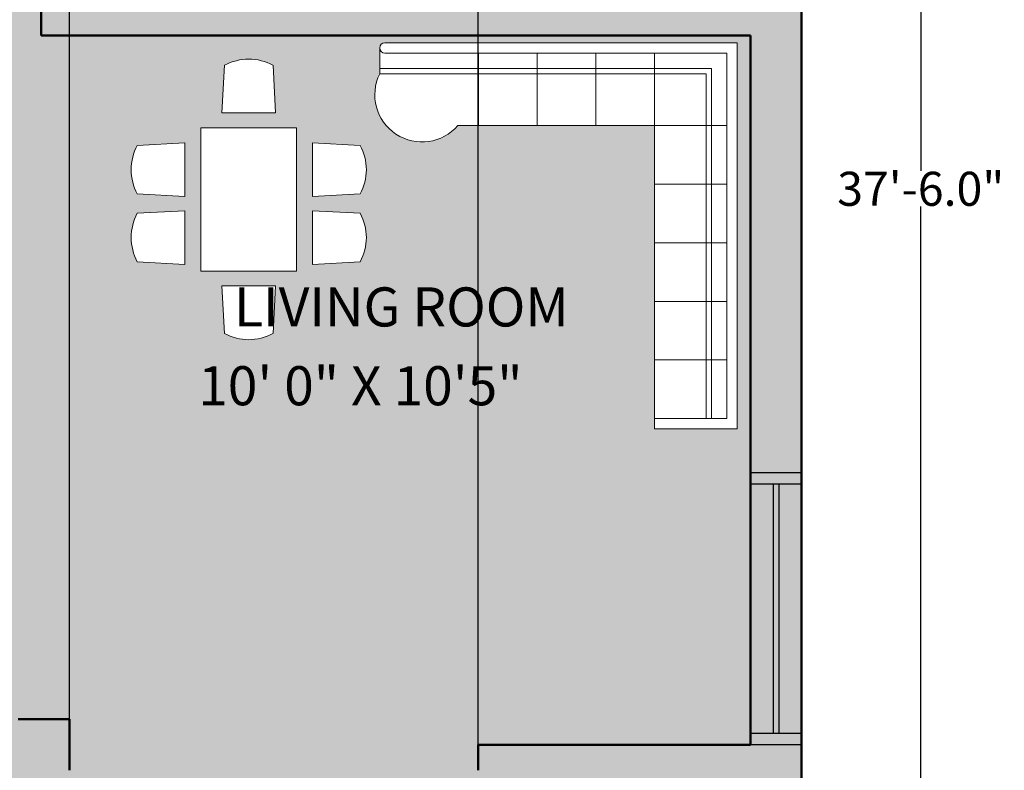
# Model space of a CAD drawing. Units: inches. Extents: x 528 to 2620, y -1066 to 798.
# Tile 24 of 41: x 1207 to 1381, y 391 to 524. Entities that reach past the tile are written whole.
import ezdxf

# ---------------------------------------------------------------- set-up
doc = ezdxf.new("R2010")
doc.units = ezdxf.units.IN
doc.header["$MEASUREMENT"] = 0
for name, color, linetype, lineweight in [('A-ANNO-DIMS', 2, 'Continuous', 18), ('A-AREA-IDEN', 7, 'Continuous', 18), ('A-FURN', 30, 'Continuous', 18), ('A-GLAZ', 3, 'Continuous', 25), ('A-WALL', 7, 'Continuous', 50), ('A-WALL-PATT', 8, 'Continuous', 13)]:
    doc.layers.add(name, color=color, linetype=linetype, lineweight=lineweight)
doc.styles.get("Standard").update_dxf_attribs({"font": 'arial.ttf'})
doc.dimstyles.get("Standard").update_dxf_attribs({"dimtxt": 6, "dimasz": 2, "dimexe": 0.18, "dimexo": 0.0625, "dimgap": 0.09, "dimtad": 0, "dimtih": 1, "dimtoh": 1, "dimdec": 1, "dimzin": 0, "dimdsep": 46, "dimlunit": 3, "dimtxsty": 'Standard', "dimblk": 'ARCHTICK', "dimcen": 0.09, "dimadec": 0, "dimazin": 0, "dimtfac": 1, "dimtdec": 1, "dimtofl": 0, "dimtmove": 0, "dimatfit": 3, "dimfxl": 1, "dimtolj": 1, "dimtzin": 0, "dimarcsym": 0})

# ---------------------------------------------------------------- blocks, each defined once
blk = doc.blocks.new('QU')
at = {"color": 0}
for p, q in [((-0.8, -2.5), (-0.8, 1.2333)), ((-0.8, 1.2333), (0, 1.2333)), ((0, 1.2333), (0, -2.4)), ((-0.7, -2.4), (-0.7, 1.1333)), ((-0.7, 1.1333), (0, 1.1333)), ((-0.55, -2.25), (-0.55, 1.1333)), ((-0.5, -2.2), (-0.5, 1.1333)), ((-0.7, 0.5666), (0, 0.5666)), ((-0.7, 0), (0, 0)), ((-0.7, -0.5667), (0, -0.5667)), ((-0.7, -1.1334), (0, -1.1334)), ((-0.7, -1.7), (1.1333, -1.7)), ((-0.1333, -1.7), (1.7, -1.7)), ((0.5667, -1.7), (0.5667, -2.4)), ((1.1333, -1.7), (1.1333, -2.4)), ((1.1334, -1.7), (1.1334, -2.4)), ((1.7, -1.7), (1.9, -1.7)), ((1.7, -1.7), (1.7, -2.4)), ((2.6553, -2.25), (-0.55, -2.25)), ((2.6553, -2.2), (-0.5, -2.2)), ((2.6553, -2.45), (2.6553, -2.2)), ((2.6053, -2.4), (-0.7, -2.4)), ((2.6053, -2.5), (-0.8, -2.5))]:
    blk.add_line(p, q, dxfattribs=at)
for centre, radius, start, end in [((2.2465, -1.9971), 0.4564, 333.59217, 139.39788), ((2.6053, -2.45), 0.05, 270, 90)]:
    blk.add_arc(centre, radius, start, end, dxfattribs=at)
blk = doc.blocks.new('table-11')
at = {"color": 0, "linetype": 'ByBlock'}
for p, q in [((-1.122, 0.5326), (-1.1442, 0.1341)), ((-0.7163, 0.5326), (-0.6942, 0.1341)), ((-0.5539, 0.5326), (-0.576, 0.1341)), ((-0.1482, 0.5326), (-0.126, 0.1341)), ((-1.1442, 0.1341), (-0.6942, 0.1341)), ((-0.576, 0.1341), (-0.126, 0.1341)), ((0, 0), (-1.2, 0)), ((-1.2, -0.8), (-1.2, 0)), ((0, -0.8), (0, 0)), ((-1.7227, -0.1971), (-1.3243, -0.175)), ((-1.3243, -0.625), (-1.3243, -0.175)), ((0.5227, -0.1971), (0.1243, -0.175)), ((0.1243, -0.625), (0.1243, -0.175)), ((-1.7227, -0.6029), (-1.3243, -0.625)), ((0.5227, -0.6029), (0.1243, -0.625)), ((0, -0.8), (-1.2, -0.8)), ((-1.1442, -0.9341), (-0.6942, -0.9341)), ((-1.122, -1.3326), (-1.1442, -0.9341)), ((-0.7163, -1.3326), (-0.6942, -0.9341)), ((-0.576, -0.9341), (-0.126, -0.9341)), ((-0.5539, -1.3326), (-0.576, -0.9341)), ((-0.1482, -1.3326), (-0.126, -0.9341))]:
    blk.add_line(p, q, dxfattribs=at)
for centre, start, end in [((-0.9192, 0.1591), 61.48912, 118.51088), ((-0.351, 0.1591), 61.48912, 118.51088), ((-1.3493, -0.4), 151.48912, 208.51088), ((0.1493, -0.4), 331.48912, 28.51088), ((-0.9192, -0.9591), 241.48912, 298.51088), ((-0.351, -0.9591), 241.48912, 298.51088)]:
    blk.add_arc(centre, 0.425, start, end, dxfattribs=at)
blk = doc.blocks.new('_ArchTick')
at = {"color": 0, "linetype": 'ByBlock', "const_width": 0.15}
blk.add_lwpolyline([(-0.5, -0.5), (0.5, 0.5)], dxfattribs=at)
blk = doc.blocks.new('*D17')
at = {"layer": 'A-ANNO-DIMS', "color": 0, "lineweight": -2, "transparency": 16777216}
for p, q in [((1345.06, 718.92), (1366.18, 718.92)), ((1366, 718.92), (1366, 497.08)), ((1366, 268.92), (1366, 490.77)), ((1345.06, 268.92), (1366.18, 268.92))]:
    blk.add_line(p, q, dxfattribs=at)
at = {"layer": 'Defpoints', "color": 0, "transparency": 16777216}
for p in [(1345, 718.92), (1345, 268.92), (1366, 268.92)]:
    blk.add_point(p, dxfattribs=at)
at = {"layer": 'A-ANNO-DIMS', "color": 0, "lineweight": -2, "transparency": 16777216, "xscale": 2, "yscale": 2, "zscale": 2}
for p, rotation in [((1366, 718.92), 90), ((1366, 268.92), 270)]:
    blk.add_blockref('_ArchTick', p, dxfattribs=dict(at, rotation=rotation))
at = {"layer": 'A-ANNO-DIMS', "color": 0, "transparency": 16777216, "insert": (1366, 493.92), "char_height": 6, "attachment_point": 5}
blk.add_mtext('\\A1;37\'-6.0"', dxfattribs=at)
blk = doc.blocks.new('WIN-1200')
for p, q in [((677.56, 718.92), (725.56, 718.92)), ((677.56, 709.92), (677.56, 718.92)), ((679.56, 709.92), (679.56, 718.92)), ((723.56, 718.92), (723.56, 709.92)), ((725.56, 718.92), (725.56, 709.92)), ((679.56, 714.92), (723.56, 714.92)), ((679.56, 713.92), (723.56, 713.92)), ((725.56, 709.92), (677.56, 709.92))]:
    blk.add_line(p, q)
blk = doc.blocks.new('*D68')
at = {"layer": 'A-ANNO-DIMS', "color": 0, "lineweight": -2, "transparency": 16777216}
for p, q in [((1216, 400.48), (1216, 751.1)), ((1216, 750.92), (1243.92, 750.92)), ((1288, 750.92), (1260.08, 750.92)), ((1288, 395.98), (1288, 751.1))]:
    blk.add_line(p, q, dxfattribs=at)
at = {"layer": 'Defpoints', "color": 0, "transparency": 16777216}
for p in [(1288, 750.92), (1216, 400.42), (1288, 395.92)]:
    blk.add_point(p, dxfattribs=at)
at = {"layer": 'A-ANNO-DIMS', "color": 0, "lineweight": -2, "transparency": 16777216, "xscale": 2, "yscale": 2, "zscale": 2, "rotation": 180}
blk.add_blockref('_ArchTick', (1216, 750.92), dxfattribs=at)
at = {"layer": 'A-ANNO-DIMS', "color": 0, "lineweight": -2, "transparency": 16777216, "xscale": 2, "yscale": 2, "zscale": 2}
blk.add_blockref('_ArchTick', (1288, 750.92), dxfattribs=at)
at = {"layer": 'A-ANNO-DIMS', "color": 0, "transparency": 16777216, "insert": (1252, 750.92), "char_height": 6, "attachment_point": 5}
blk.add_mtext('\\A1;6\'-0"', dxfattribs=at)

msp = doc.modelspace()

# ---------------------------------------------------------------- hatches: boundary and pattern name
at = {"layer": 'A-WALL-PATT', "transparency": 33554521}
h = msp.add_hatch(color=256, dxfattribs=at)
h.dxf.hatch_style = 1
h.paths.add_polyline_path([(1066, 709.92), (1114.5, 709.92), (1114.5, 718.92), (1057, 718.92), (1057, 667.92), (1066, 667.92)])
h.paths.add_polyline_path([(1227.5, 718.92), (1162.5, 718.92), (1162.5, 709.92), (1211, 709.92), (1211, 577.92), (1205.42, 577.92), (1205.5, 573.42), (1211, 573.42), (1211, 567.42), (1215.5, 567.42), (1215.5, 669.42), (1268, 669.42), (1268, 675.92), (1263.5, 675.92), (1263.5, 673.92), (1215.5, 673.92), (1215.5, 709.92), (1227.5, 709.92)])
h.paths.add_polyline_path([(1345, 718.92), (1316, 718.92), (1316, 709.92), (1336, 709.92), (1336, 641.67), (1345, 641.67)])
h.paths.add_polyline_path([(1066, 619.92), (1057, 619.92), (1057, 561.42), (1066, 561.42), (1066, 573.42), (1161, 573.42), (1161, 569.42), (1165.5, 569.42), (1165.5, 577.92), (1066, 577.92)])
h.paths.add_polyline_path([(1216, 391.42), (1216, 400.42), (1207, 400.42), (1201, 400.42), (1201, 397.42), (1201, 391.42), (1207, 391.42), (1207, 268.92), (1252, 268.92), (1252, 277.92), (1216, 277.92), (1216, 359.77)])
h.paths.add_polyline_path([(1345, 395.92), (1336, 395.92), (1288, 395.92), (1288, 391.42), (1336, 391.42), (1336, 277.92), (1300, 277.92), (1300, 268.92), (1345, 268.92)])
h.paths.add_polyline_path([(1345, 593.67), (1336, 593.67), (1336, 525.42), (1215.5, 525.42), (1215.5, 527.17), (1211, 527.17), (1211, 520.92), (1336, 520.92), (1336, 443.92), (1345, 443.92)])
h.paths.add_polyline_path([(1066, 520.92), (1165.5, 520.92), (1165.5, 545.42), (1161, 545.42), (1161, 525.42), (1066, 525.42), (1066, 537.42), (1057, 537.42), (1057, 484.67), (1066, 484.67)])
h.paths.add_polyline_path([(1066, 436.67), (1057, 436.67), (1057, 391.42), (1085.5, 391.42), (1085.5, 400.42), (1066, 400.42)])
h.paths.add_polyline_path([(1153, 397.42), (1153, 400.42), (1133.5, 400.42), (1133.5, 391.42), (1153, 391.42)])
at = {"layer": 'A-WALL-PATT', "transparency": 33554681}
h = msp.add_hatch(color=256, dxfattribs=at)
h.dxf.hatch_style = 1
h.paths.add_polyline_path([(1066, 665.92), (1062, 665.92), (1062, 621.92), (1066, 621.92)])
h.paths.add_polyline_path([(1061, 665.92), (1057, 665.92), (1057, 621.92), (1061, 621.92)])
h.paths.add_polyline_path([(1160.5, 713.92), (1116.5, 713.92), (1116.5, 709.92), (1160.5, 709.92)])
h.paths.add_polyline_path([(1160.5, 718.92), (1116.5, 718.92), (1116.5, 714.92), (1160.5, 714.92)])
h.paths.add_polyline_path([(1251.5, 713.92), (1227.5, 713.92), (1227.5, 709.92), (1251.5, 709.92)])
h.paths.add_polyline_path([(1251.5, 718.92), (1227.5, 718.92), (1227.5, 714.92), (1251.5, 714.92)])
h.paths.add_polyline_path([(1314, 713.92), (1270, 713.92), (1270, 709.92), (1314, 709.92)])
h.paths.add_polyline_path([(1314, 718.92), (1270, 718.92), (1270, 714.92), (1314, 714.92)])
h.paths.add_polyline_path([(1345, 639.67), (1341, 639.67), (1341, 595.67), (1345, 595.67)])
h.paths.add_polyline_path([(1340, 639.67), (1336, 639.67), (1336, 595.67), (1340, 595.67)])
h.paths.add_polyline_path([(1345, 441.92), (1341, 441.92), (1341, 397.92), (1345, 397.92)])
h.paths.add_polyline_path([(1340, 441.92), (1336, 441.92), (1336, 397.92), (1340, 397.92)])
h.paths.add_polyline_path([(1298, 272.92), (1254, 272.92), (1254, 268.92), (1298, 268.92)])
h.paths.add_polyline_path([(1298, 277.92), (1254, 277.92), (1254, 273.92), (1298, 273.92)])
h.paths.add_polyline_path([(1131.5, 395.42), (1087.5, 395.42), (1087.5, 391.42), (1131.5, 391.42)])
h.paths.add_polyline_path([(1131.5, 400.42), (1087.5, 400.42), (1087.5, 396.42), (1131.5, 396.42)])
h.paths.add_polyline_path([(1066, 482.67), (1062, 482.67), (1062, 438.67), (1066, 438.67)])
h.paths.add_polyline_path([(1061, 482.67), (1057, 482.67), (1057, 438.67), (1061, 438.67)])
h.paths.add_polyline_path([(1066, 561.42), (1062, 561.42), (1062, 537.42), (1066, 537.42)])
h.paths.add_polyline_path([(1061, 561.42), (1057, 561.42), (1057, 537.42), (1061, 537.42)])
at = {"layer": 'A-WALL-PATT', "transparency": 33554536}
h = msp.add_hatch(color=256, dxfattribs=at)
h.dxf.hatch_style = 1
h.paths.add_polyline_path([(1336, 709.92), (1268, 709.92), (1268, 699.92), (1266.75, 699.92), (1266.75, 675.92), (1268, 675.92), (1268, 669.42), (1215.5, 669.42), (1215.5, 567.17), (1217, 567.17), (1257, 567.17), (1257, 565.42), (1256.96, 565.42, -0.401453), (1217, 527.17), (1215.5, 527.17), (1215.5, 525.42), (1336, 525.42)], flags=17)
h.paths.add_polyline_path([(1285.03, 635.93), (1285.23, 636.13), (1285.67, 636.26), (1286.21, 636.02), (1286.98, 636.08), (1332.98, 636.08), (1333.36, 636.22), (1333.82, 636.08), (1334.11, 635.71), (1334.11, 635.3), (1333.91, 634.86), (1333.82, 634.83), (1333.82, 592.74), (1333.97, 592.6), (1334.11, 592.29), (1334.11, 591.88), (1333.82, 591.51), (1333.36, 591.37), (1332.98, 591.51), (1332.64, 591.79), (1332.64, 591.51), (1286.98, 591.51), (1286.17, 591.67), (1286.07, 591.57), (1285.68, 591.37), (1285.23, 591.51), (1285.03, 591.71), (1284.83, 592.1), (1284.98, 592.54), (1285.13, 592.69), (1285.13, 634.95), (1284.98, 635.1), (1284.83, 635.54)], flags=16)
h.paths.add_polyline_path([(1285.03, 635.93), (1285.23, 636.13), (1285.67, 636.26), (1286.21, 636.02), (1286.98, 636.08), (1332.98, 636.08), (1333.36, 636.22), (1333.82, 636.08), (1334.11, 635.71), (1334.11, 635.3), (1333.97, 634.99), (1333.82, 634.85), (1333.82, 592.74), (1333.97, 592.6), (1334.11, 592.29), (1334.11, 591.88), (1333.82, 591.51), (1333.36, 591.37), (1332.98, 591.51), (1332.64, 591.79), (1332.64, 592.25), (1332.64, 635.35), (1332.64, 635.8), (1332.98, 636.08), (1312.23, 636.08), (1311.1, 635.48), (1310.63, 635.48), (1310.43, 635.23), (1309.94, 635.1), (1309.7, 634.99), (1309.06, 634.76), (1308.71, 634.61), (1308.32, 634.61), (1307.75, 634.36), (1307.11, 634.27), (1307.01, 634.11), (1306.77, 634.02), (1307.25, 633.28), (1306.87, 633.04), (1306.77, 632.88), (1306.37, 632.64), (1306.03, 632.55), (1305.54, 632.41), (1315.47, 618.49), (1316.32, 619.39), (1312.77, 622.86), (1319.62, 630.11), (1320.07, 629.68), (1320.11, 630), (1320.28, 630.6), (1320.53, 631.18), (1320.53, 632.01), (1320.26, 632.55), (1320.11, 633.13), (1320.06, 633.73), (1320.63, 634.02), (1321.22, 634.16), (1321.86, 634.11), (1322.45, 633.91), (1322.99, 633.62), (1324.1, 633.62), (1324.64, 633.91), (1325.23, 634.07), (1325.87, 634.07), (1326.43, 633.91), (1326.98, 633.62), (1328.35, 633.62), (1328.9, 633.91), (1329.49, 634.11), (1330.1, 634.16), (1330.69, 634.02), (1331.28, 633.73), (1331.23, 633.13), (1331.09, 632.55), (1330.79, 632.01), (1330.79, 631.18), (1331.04, 630.6), (1331.23, 630), (1331.28, 629.41), (1331.19, 628.79), (1331.04, 628.18), (1330.79, 627.6), (1330.79, 626.77), (1331.04, 626.19), (1331.23, 625.59), (1331.28, 625.01), (1331.19, 624.38), (1331.04, 623.78), (1330.79, 623.24), (1330.79, 622.37), (1331.04, 621.83), (1331.23, 621.25), (1331.28, 620.6), (1331.19, 619.97), (1331.04, 619.37), (1330.79, 618.83), (1330.79, 617.96), (1331.09, 617.42), (1331.23, 616.88), (1331.28, 616.23), (1331.28, 615.52), (1330.69, 615.27), (1330.1, 615.12), (1329.49, 615.12), (1328.9, 615.32), (1328.35, 615.65), (1326.98, 615.65), (1326.43, 615.32), (1325.87, 615.16), (1325.23, 615.16), (1324.64, 615.32), (1324.1, 615.65), (1323.24, 615.65), (1324.93, 614.04), (1322.98, 611.98), (1324.1, 611.98), (1324.64, 612.27), (1325.28, 612.43), (1325.87, 612.43), (1326.48, 612.27), (1327.03, 611.98), (1328.35, 611.98), (1328.9, 612.27), (1329.49, 612.48), (1330.1, 612.52), (1330.74, 612.39), (1331.28, 612.07), (1331.28, 611.36), (1331.28, 610.75), (1331.09, 610.17), (1330.79, 609.63), (1330.79, 608.81), (1331.09, 608.22), (1331.23, 607.62), (1331.28, 606.99), (1331.23, 606.41), (1331.09, 605.81), (1330.79, 605.22), (1330.79, 604.4), (1331.09, 603.81), (1331.23, 603.21), (1331.28, 602.63), (1331.23, 602), (1331.09, 601.4), (1330.79, 600.86), (1330.79, 599.99), (1331.09, 599.45), (1331.23, 598.87), (1331.28, 598.22), (1331.23, 597.59), (1331.09, 596.99), (1330.79, 596.45), (1330.79, 595.58), (1331.09, 595.04), (1331.28, 594.51), (1331.28, 593.86), (1330.74, 593.61), (1330.1, 593.48), (1329.49, 593.48), (1328.9, 593.68), (1328.35, 594.01), (1327.03, 594.01), (1326.48, 593.68), (1325.87, 593.52), (1325.28, 593.52), (1324.64, 593.68), (1324.1, 594.01), (1323.04, 594.01), (1322.5, 593.68), (1321.91, 593.48), (1321.27, 593.48), (1320.63, 593.61), (1320.11, 593.86), (1320.11, 594.51), (1320.28, 595.04), (1320.58, 595.58), (1320.58, 596.45), (1320.28, 596.99), (1320.16, 597.59), (1320.1, 598.01), (1319.62, 597.55), (1315.66, 601.73), (1312.23, 591.57), (1311.74, 591.66), (1311.59, 591.91), (1310.78, 592.4), (1309.55, 592.89), (1308.96, 592.89), (1308.71, 593.03), (1308.56, 593.14), (1307.75, 593.52), (1306.77, 593.61), (1307.25, 594.36), (1306.87, 594.6), (1306.37, 594.84), (1306.03, 595.09), (1305.54, 595.24), (1315.46, 609.35), (1310.93, 613.71), (1315.47, 618.49), (1305.54, 632.41), (1306.03, 632.55), (1306.37, 632.64), (1306.77, 632.88), (1306.87, 633.04), (1307.25, 633.28), (1306.77, 634.02), (1307.01, 634.11), (1307.11, 634.27), (1307.75, 634.36), (1308.32, 634.61), (1308.71, 634.61), (1309.06, 634.76), (1309.7, 634.99), (1309.94, 635.1), (1310.43, 635.23), (1310.63, 635.48), (1311.1, 635.48), (1312.23, 636.08), (1286.98, 636.08), (1286.22, 636.02), (1286.41, 635.44), (1286.21, 635.05), (1286.02, 634.85), (1285.87, 634.81), (1285.87, 592.84), (1286.15, 592.73), (1286.41, 592.19), (1286.23, 591.66), (1286.17, 591.67), (1286.07, 591.57), (1285.68, 591.37), (1285.23, 591.51), (1285.03, 591.71), (1284.83, 592.1), (1284.98, 592.54), (1285.13, 592.69), (1285.13, 634.95), (1284.98, 635.1), (1284.83, 635.54)], flags=0)
h.paths.add_polyline_path([(1322.5, 653.6), (1333.65, 653.6), (1333.65, 637.99), (1322.5, 637.99)], flags=16)
h.paths.add_polyline_path([(1323.62, 652.48), (1332.53, 652.48), (1332.53, 639.11), (1323.62, 639.11)], flags=0)
edge = h.paths.add_edge_path(flags=0)
edge.add_ellipse((1328.07, 645.79), major_axis=(2.24, 2.24), ratio=1, start_angle=405, end_angle=495, ccw=False)
edge.add_ellipse((1328.07, 645.79), major_axis=(2.24, 2.24), ratio=1, start_angle=675, end_angle=765, ccw=False)
edge.add_ellipse((1328.07, 645.79), major_axis=(2.24, 2.24), ratio=1, start_angle=585, end_angle=675, ccw=False)
edge.add_ellipse((1328.07, 645.79), major_axis=(2.24, 2.24), ratio=1, start_angle=495, end_angle=585, ccw=False)
h.paths.add_polyline_path([(1320.58, 628.39), (1320.33, 628.01), (1320.61, 628.55)], flags=0)
h.paths.add_polyline_path([(1317.89, 604.89), (1318.78, 604.64), (1319.76, 604.28), (1318.88, 604.53)], flags=0)
h.paths.add_polyline_path([(1320.33, 599.65), (1320.58, 599.25), (1320.58, 599.16)], flags=0)
h.paths.add_polyline_path([(1322.5, 589.6), (1333.65, 589.6), (1333.65, 573.99), (1322.5, 573.99)], flags=16)
h.paths.add_polyline_path([(1323.62, 588.48), (1332.53, 588.48), (1332.53, 575.11), (1323.62, 575.11)], flags=0)
edge = h.paths.add_edge_path(flags=0)
edge.add_ellipse((1328.07, 581.8), major_axis=(-2.24, 2.24), ratio=1, start_angle=-45, end_angle=45, ccw=False)
edge.add_ellipse((1328.07, 581.8), major_axis=(-2.24, 2.24), ratio=1, start_angle=-135, end_angle=-45, ccw=False)
edge.add_ellipse((1328.07, 581.8), major_axis=(-2.24, 2.24), ratio=1, start_angle=135, end_angle=-135, ccw=False)
edge.add_ellipse((1328.07, 581.8), major_axis=(-2.24, 2.24), ratio=1, start_angle=45, end_angle=135, ccw=False)
h.paths.add_polyline_path([(1264.75, 699.92), (1263.5, 699.92), (1263.5, 709.92), (1215.5, 709.92), (1215.5, 673.92), (1263.5, 673.92), (1263.5, 675.92), (1264.75, 675.92)], flags=16)
h.paths.add_polyline_path([(1162.19, 569.42), (1161, 569.42), (1161, 573.42), (1066, 573.42), (1066, 525.42), (1161, 525.42), (1161, 545.42), (1162.19, 545.42)])
h.paths.add_polyline_path([(1256.96, 565.42), (1257, 565.42), (1257, 567.17), (1217, 567.17), (1215.5, 567.17), (1215.5, 567.42), (1211, 567.42), (1211, 573.42), (1205.5, 573.42), (1205.42, 577.92), (1211, 577.92), (1211, 709.92), (1066, 709.92), (1066, 577.92), (1165.5, 577.92), (1165.5, 569.42), (1164.19, 569.42), (1164.19, 545.42), (1165.5, 545.42), (1165.5, 520.92), (1153, 520.92), (1153, 484.92), (1102, 484.92), (1102, 436.42), (1153, 436.42), (1153, 400.42), (1153, 391.42), (1201, 391.42), (1201, 400.42), (1207, 400.42), (1216, 400.42), (1216, 391.42), (1216, 277.92), (1336, 277.92), (1336, 391.42), (1288, 391.42), (1288, 395.92), (1336, 395.92), (1336, 443.92), (1336, 520.92), (1211, 520.92), (1211, 527.17), (1215.5, 527.17), (1217, 527.17, 0.401453)])
h.paths.add_polyline_path([(1167.25, 579.42), (1165.5, 579.42), (1165.5, 619.42), (1167.25, 619.42)], flags=16)
h.paths.add_polyline_path([(1227.97, 501.56), (1236.36, 502.03), (1236.36, 492.55), (1227.97, 493.02, -0.254069)], flags=16)
h.paths.add_polyline_path([(1243.34, 515.69, -0.254069), (1251.88, 515.69), (1252.35, 507.3), (1242.87, 507.3)], flags=16)
h.paths.add_polyline_path([(1239.18, 504.68), (1256.03, 504.68), (1256.03, 479.42), (1239.18, 479.42)], flags=16)
h.paths.add_polyline_path([(1227.97, 489.6), (1236.36, 490.07), (1236.36, 480.59), (1227.97, 481.06, -0.254069)], flags=16)
h.paths.add_polyline_path([(1197.2, 624.04), (1197.2, 639.64), (1208.35, 639.64), (1208.35, 624.04)], flags=16)
h.paths.add_polyline_path([(1198.32, 625.15), (1198.32, 638.53), (1207.23, 638.53), (1207.23, 625.15)], flags=0)
h.paths.add_polyline_path([(1258.85, 502.03), (1267.25, 501.56, -0.254069), (1267.25, 493.02), (1258.85, 492.55)], flags=16)
h.paths.add_polyline_path([(1271.59, 519.66), (1333.67, 519.66), (1333.67, 451.59), (1319.09, 451.59), (1319.09, 505.07), (1288.09, 505.07), (1284.45, 505.07, -0.883215), (1270.68, 514.19), (1270.68, 518.75, -0.414214)], flags=16)
h.paths.add_polyline_path([(1331.85, 517.83), (1331.85, 453.42), (1328.2, 453.42), (1328.2, 505.07), (1298.42, 505.07), (1298.42, 514.19), (1288.09, 514.19), (1288.09, 517.83)], flags=0)
h.paths.add_polyline_path([(1242.87, 476.8), (1252.35, 476.8), (1251.88, 468.41, -0.254069), (1243.34, 468.41)], flags=16)
h.paths.add_polyline_path([(1258.85, 490.07), (1267.25, 489.6, -0.254069), (1267.25, 481.06), (1258.85, 480.59)], flags=16)
h.paths.add_polyline_path([(1161.68, 641.55), (1160.87, 641.72), (1160.77, 641.62), (1160.38, 641.41), (1159.93, 641.55), (1159.73, 641.75), (1159.53, 642.14), (1159.68, 642.58), (1159.83, 642.73), (1159.83, 684.99), (1159.68, 685.14), (1159.53, 685.58), (1159.73, 685.97), (1159.93, 686.17), (1160.37, 686.31), (1160.91, 686.06), (1161.68, 686.13), (1207.68, 686.13), (1208.06, 686.27), (1208.52, 686.13), (1208.81, 685.76), (1208.81, 685.34), (1208.61, 684.9), (1208.52, 684.87), (1208.52, 642.78), (1208.67, 642.65), (1208.88, 642.2), (1208.72, 641.8), (1208.52, 641.55), (1208.06, 641.41), (1207.68, 641.55), (1207.34, 641.83), (1207.34, 641.55)], flags=16)
h.paths.add_polyline_path([(1186.93, 641.62), (1186.44, 641.71), (1186.29, 641.95), (1185.48, 642.45), (1184.25, 642.94), (1183.66, 642.94), (1183.41, 643.07), (1183.26, 643.18), (1182.45, 643.57), (1181.47, 643.65), (1181.95, 644.4), (1181.57, 644.64), (1181.07, 644.89), (1180.73, 645.13), (1180.24, 645.29), (1190.16, 659.4), (1185.63, 663.75), (1190.17, 668.54), (1180.24, 682.46), (1180.73, 682.59), (1181.07, 682.68), (1181.47, 682.93), (1181.57, 683.08), (1181.95, 683.33), (1181.47, 684.07), (1181.71, 684.16), (1181.81, 684.31), (1182.45, 684.4), (1183.02, 684.65), (1183.41, 684.65), (1183.76, 684.81), (1184.4, 685.03), (1184.64, 685.14), (1185.13, 685.28), (1185.33, 685.52), (1185.8, 685.52), (1186.93, 686.13), (1161.68, 686.13), (1160.92, 686.06), (1161.11, 685.49), (1160.91, 685.1), (1160.72, 684.9), (1160.57, 684.85), (1160.57, 642.88), (1160.85, 642.77), (1161.11, 642.23), (1160.93, 641.7), (1160.87, 641.72), (1160.77, 641.62), (1160.38, 641.41), (1159.93, 641.55), (1159.73, 641.75), (1159.53, 642.14), (1159.68, 642.58), (1159.83, 642.73), (1159.83, 684.99), (1159.68, 685.14), (1159.53, 685.58), (1159.73, 685.97), (1159.93, 686.17), (1160.37, 686.31), (1160.91, 686.06), (1161.68, 686.13), (1207.68, 686.13), (1208.06, 686.27), (1208.52, 686.13), (1208.81, 685.76), (1208.81, 685.34), (1208.67, 685.03), (1208.52, 684.9), (1208.52, 642.78), (1208.67, 642.65), (1208.88, 642.2), (1208.72, 641.8), (1208.52, 641.55), (1208.06, 641.41), (1207.68, 641.55), (1207.34, 641.83), (1207.34, 642.29), (1207.34, 685.39), (1207.34, 685.85), (1207.68, 686.13), (1186.93, 686.13), (1185.8, 685.52), (1185.33, 685.52), (1185.13, 685.28), (1184.64, 685.14), (1184.4, 685.03), (1183.76, 684.81), (1183.41, 684.65), (1183.02, 684.65), (1182.45, 684.4), (1181.81, 684.31), (1181.71, 684.16), (1181.47, 684.07), (1181.95, 683.33), (1181.57, 683.08), (1181.47, 682.93), (1181.07, 682.68), (1180.73, 682.59), (1180.24, 682.46), (1190.17, 668.54), (1191.02, 669.43), (1187.47, 672.9), (1194.32, 680.15), (1194.77, 679.72), (1194.81, 680.04), (1194.98, 680.65), (1195.23, 681.23), (1195.23, 682.05), (1194.96, 682.59), (1194.81, 683.17), (1194.76, 683.78), (1195.33, 684.07), (1195.92, 684.2), (1196.56, 684.16), (1197.15, 683.96), (1197.69, 683.67), (1198.8, 683.67), (1199.34, 683.96), (1199.93, 684.11), (1200.57, 684.11), (1201.13, 683.96), (1201.68, 683.67), (1203.05, 683.67), (1203.6, 683.96), (1204.19, 684.16), (1204.8, 684.2), (1205.39, 684.07), (1205.98, 683.78), (1205.93, 683.17), (1205.79, 682.59), (1205.49, 682.05), (1205.49, 681.23), (1205.74, 680.65), (1205.93, 680.04), (1205.98, 679.46), (1205.89, 678.83), (1205.74, 678.23), (1205.49, 677.65), (1205.49, 676.82), (1205.74, 676.24), (1205.93, 675.63), (1205.98, 675.05), (1205.89, 674.42), (1205.74, 673.82), (1205.49, 673.28), (1205.49, 672.41), (1205.74, 671.87), (1205.93, 671.29), (1205.98, 670.64), (1205.89, 670.02), (1205.74, 669.41), (1205.49, 668.87), (1205.49, 668), (1205.79, 667.46), (1205.93, 666.93), (1205.98, 666.28), (1205.98, 665.56), (1205.39, 665.32), (1204.8, 665.16), (1204.19, 665.16), (1203.6, 665.36), (1203.05, 665.7), (1201.68, 665.7), (1201.13, 665.36), (1200.57, 665.2), (1199.93, 665.2), (1199.34, 665.36), (1198.8, 665.7), (1197.94, 665.7), (1199.63, 664.09), (1197.68, 662.03), (1198.8, 662.03), (1199.34, 662.32), (1199.98, 662.47), (1200.57, 662.47), (1201.18, 662.32), (1201.73, 662.03), (1203.05, 662.03), (1203.6, 662.32), (1204.19, 662.52), (1204.8, 662.56), (1205.44, 662.43), (1205.98, 662.12), (1205.98, 661.4), (1205.98, 660.8), (1205.79, 660.21), (1205.49, 659.68), (1205.49, 658.85), (1205.79, 658.27), (1205.93, 657.66), (1205.98, 657.04), (1205.93, 656.45), (1205.79, 655.85), (1205.49, 655.27), (1205.49, 654.44), (1205.79, 653.86), (1205.93, 653.25), (1205.98, 652.67), (1205.93, 652.05), (1205.79, 651.44), (1205.49, 650.91), (1205.49, 650.03), (1205.79, 649.5), (1205.93, 648.91), (1205.98, 648.26), (1205.93, 647.64), (1205.79, 647.03), (1205.49, 646.5), (1205.49, 645.62), (1205.79, 645.09), (1205.98, 644.55), (1205.98, 643.9), (1205.44, 643.65), (1204.8, 643.52), (1204.19, 643.52), (1203.6, 643.72), (1203.05, 644.06), (1201.73, 644.06), (1201.18, 643.72), (1200.57, 643.57), (1199.98, 643.57), (1199.34, 643.72), (1198.8, 644.06), (1197.74, 644.06), (1197.2, 643.72), (1196.61, 643.52), (1195.97, 643.52), (1195.33, 643.65), (1194.81, 643.9), (1194.81, 644.55), (1194.98, 645.09), (1195.28, 645.62), (1195.28, 646.5), (1194.98, 647.03), (1194.86, 647.64), (1194.8, 648.06), (1194.32, 647.59), (1190.36, 651.77)], flags=16)
h.paths.add_polyline_path([(1195.28, 649.2), (1195.03, 649.7), (1195.28, 649.29)], flags=0)
h.paths.add_polyline_path([(1194.46, 654.33), (1193.58, 654.58), (1192.59, 654.93), (1193.48, 654.69)], flags=0)
h.paths.add_polyline_path([(1195.28, 678.43), (1195.03, 678.05), (1195.31, 678.59)], flags=0)
h.paths.add_polyline_path([(1197.2, 688.04), (1197.2, 703.64), (1208.35, 703.64), (1208.35, 688.04)], flags=16)
h.paths.add_polyline_path([(1198.32, 689.15), (1198.32, 702.53), (1207.23, 702.53), (1207.23, 689.15)], flags=0)
h.paths.add_polyline_path([(1217.1, 329.02), (1230.65, 329.02), (1230.65, 315.47), (1217.1, 315.47)], flags=16)
h.paths.add_polyline_path([(1223.87, 322.24), (1227.26, 322.24), (1227.26, 321.32, -0.414214), (1229.73, 318.86, -1), (1224.8, 318.86), (1223.87, 318.86)], flags=0)
h.paths.add_polyline_path([(1222.11, 325.63, -1), (1218.86, 325.63, -1)], flags=0)
h.paths.add_polyline_path([(1228.25, 325.63, -1), (1226.28, 325.63, -1)], flags=0)
h.paths.add_polyline_path([(1221.53, 318.86, -1), (1219.44, 318.86, -1)], flags=0)
h.paths.add_polyline_path([(1299.15, 293.73), (1299.15, 278.54), (1271.23, 278.54), (1271.23, 293.73)], flags=16)
h.paths.add_polyline_path([(1259.69, 292.21), (1270.62, 292.21, -1), (1270.62, 291.6), (1259.69, 291.6, -1)], flags=16)
h.paths.add_polyline_path([(1259.69, 291.3), (1270.62, 291.3, -1), (1270.62, 290.69), (1259.69, 290.69, -1)], flags=16)
h.paths.add_polyline_path([(1259.69, 290.39), (1270.62, 290.39, -1), (1270.62, 289.78), (1259.69, 289.78, -1)], flags=16)
h.paths.add_polyline_path([(1259.69, 289.48), (1270.62, 289.48, -1), (1270.62, 288.87), (1259.69, 288.87, -1)], flags=16)
h.paths.add_polyline_path([(1259.69, 288.57), (1270.62, 288.57, -1), (1270.62, 287.96), (1259.69, 287.96, -1)], flags=16)
h.paths.add_polyline_path([(1274.41, 292.38), (1283.25, 292.38, -0.414214), (1285.07, 290.56), (1285.07, 283.64, -0.414214), (1283.25, 281.82), (1277.72, 281.82), (1278.67, 280.87, -0.57735), (1279.38, 280.16), (1279.44, 280.11, -1), (1279.03, 279.7), (1278.97, 279.75, -0.57735), (1278.26, 280.46), (1276.9, 281.82), (1274.41, 281.82, -0.414214), (1272.58, 283.64), (1272.58, 290.56, -0.414214)], flags=0)
h.paths.add_polyline_path([(1259.69, 287.65), (1270.62, 287.65, -1), (1270.62, 287.05), (1259.69, 287.05, -1)], flags=16)
h.paths.add_polyline_path([(1259.69, 286.74), (1270.62, 286.74, -1), (1270.62, 286.14), (1259.69, 286.14, -1)], flags=16)
h.paths.add_polyline_path([(1259.69, 285.83), (1270.62, 285.83, -1), (1270.62, 285.22), (1259.69, 285.22, -1)], flags=16)
h.paths.add_polyline_path([(1259.69, 284.92), (1270.62, 284.92, -1), (1270.62, 284.31), (1259.69, 284.31, -1)], flags=16)
h.paths.add_polyline_path([(1259.69, 284.01), (1270.62, 284.01, -1), (1270.62, 283.4), (1259.69, 283.4, -1)], flags=16)
h.paths.add_polyline_path([(1287.82, 292.38), (1296.67, 292.38, -0.414214), (1298.49, 290.56), (1298.49, 283.64, -0.414214), (1296.67, 281.82), (1291.14, 281.82), (1292.09, 280.87, -0.57735), (1292.8, 280.16), (1292.85, 280.11, -1), (1292.44, 279.7), (1292.39, 279.75, -0.57735), (1291.68, 280.46), (1290.32, 281.82), (1287.82, 281.82, -0.414214), (1286, 283.64), (1286, 290.56, -0.414214)], flags=0)
h.paths.add_polyline_path([(1259.69, 283.1), (1270.62, 283.1, -1), (1270.62, 282.49), (1259.69, 282.49, -1)], flags=16)
h.paths.add_polyline_path([(1279.94, 287.61, -1), (1278.01, 287.61, -1)], flags=0)
h.paths.add_polyline_path([(1259.69, 282.19), (1270.62, 282.19, -1), (1270.62, 281.58), (1259.69, 281.58, -1)], flags=16)
h.paths.add_polyline_path([(1259.69, 281.27), (1270.62, 281.27, -1), (1270.62, 280.67), (1259.69, 280.67, -1)], flags=16)
h.paths.add_polyline_path([(1275.16, 284.17, -1), (1274.77, 284.17, -1)], flags=0)
h.paths.add_polyline_path([(1293.36, 287.61, -1), (1291.43, 287.61, -1)], flags=0)
h.paths.add_polyline_path([(1275.14, 280.5), (1276.33, 280.5, -5.828427), (1276.33, 280.12), (1275.14, 280.12, -1)], flags=0)
h.paths.add_polyline_path([(1288.57, 284.17, -1), (1288.19, 284.17, -1)], flags=0)
h.paths.add_polyline_path([(1281.31, 280.5), (1282.5, 280.5, -1), (1282.5, 280.12), (1281.31, 280.12, -5.828427)], flags=0)
h.paths.add_polyline_path([(1288.56, 280.5), (1289.75, 280.5, -5.828427), (1289.75, 280.12), (1288.56, 280.12, -1)], flags=0)
h.paths.add_polyline_path([(1294.73, 280.5), (1295.92, 280.5, -1), (1295.92, 280.12), (1294.73, 280.12, -5.828427)], flags=0)
h.paths.add_polyline_path([(1207, 391.42), (1201, 391.42), (1061.5, 391.42), (1061.5, 307.96), (1069, 307.96), (1069, 305.42), (1207, 305.42)])
h = msp.add_hatch(color=256, dxfattribs=at)
h.dxf.hatch_style = 1
h.paths.add_polyline_path([(1340, 441.92), (1336, 441.92), (1336, 397.92), (1340, 397.92)])
h.paths.add_polyline_path([(1345, 443.92), (1336, 443.92), (1336, 441.92), (1340, 441.92), (1345, 441.92)])
h.paths.add_polyline_path([(1345, 397.92), (1336, 397.92), (1336, 395.92), (1345, 395.92)])
h.paths.add_polyline_path([(1341, 441.92), (1340, 441.92), (1340, 397.92), (1341, 397.92)])
h.paths.add_polyline_path([(1345, 595.67), (1336, 595.67), (1336, 593.67), (1345, 593.67)])
h.paths.add_polyline_path([(1345, 641.67), (1336, 641.67), (1336, 639.67), (1345, 639.67)])
h.paths.add_polyline_path([(1341, 639.67), (1340, 639.67), (1340, 595.67), (1341, 595.67)])
h.paths.add_polyline_path([(1062, 561.42), (1061, 561.42), (1061, 537.42), (1062, 537.42)])

# ---------------------------------------------------------------- linework, layer by layer
at = {"layer": 'A-WALL'}
for p, q in [((1345, 268.92), (1345, 718.92)), ((1211, 527.17), (1211, 520.92)), ((1336, 520.92), (1211, 520.92)), ((1336, 395.92), (1336, 520.92)), ((1216, 400.42), (1207, 400.42)), ((1216, 391.42), (1216, 400.42)), ((1336, 395.92), (1288, 395.92)), ((1288, 395.92), (1288, 391.42))]:
    msp.add_line(p, q, dxfattribs=at)

# ---------------------------------------------------------------- block references
at = {"layer": 'A-FURN'}
for name, p, xscale, yscale, zscale, rotation in [('QU', (1319.09, 474.08), 18.23103046096107, 18.23103046096107, 18.23103046096107, 180), ('table-11', (1239.18, 504.68), 21.05693885866703, 21.05693885866703, 21.05693885866703, 90)]:
    msp.add_blockref(name, p, dxfattribs=dict(at, xscale=xscale, yscale=yscale, zscale=zscale, rotation=rotation))
at = {"layer": 'A-GLAZ', "rotation": 270.0000000000007}
msp.add_blockref('WIN-1200', (626.07, 1121.48), dxfattribs=at)

# ---------------------------------------------------------------- texts
at = {"layer": 'A-AREA-IDEN'}
for s, p in [('LIVING ROOM', (1245.02, 469.65)), ('10\' 0" X 10\'5"', (1238.69, 455.76))]:
    msp.add_text(s, height=6.8907, dxfattribs=at).set_placement(p)

# ---------------------------------------------------------------- dimensions: what is measured, and where the dimension line sits
at = {"layer": 'A-ANNO-DIMS'}
dim = msp.add_linear_dim(base=(1288, 750.92), p1=(1216, 400.42), p2=(1288, 395.92), dimstyle='Standard', override={"dimdec": 1, "dimlfac": 1, "dimrnd": 0, "dimzin": 1, "dimdsep": 46, "dimlunit": 4, "dimfrac": 2}, dxfattribs=at)
dim.commit()
dim.dimension.update_dxf_attribs({"geometry": '*D68', "text_midpoint": (1252, 750.92)})
dim = msp.add_linear_dim(base=(1366, 268.92), p1=(1345, 718.92), p2=(1345, 268.92), angle=90, dimstyle='Standard', override={"dimclrd": 0, "dimclre": 0, "dimclrt": 0}, dxfattribs=at)
dim.commit()
dim.dimension.update_dxf_attribs({"geometry": '*D17', "text_midpoint": (1366, 493.92)})

doc.saveas('drawing.dxf')
